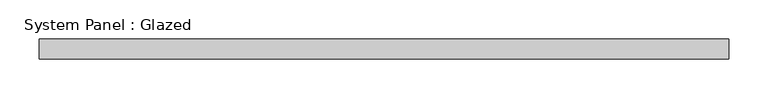
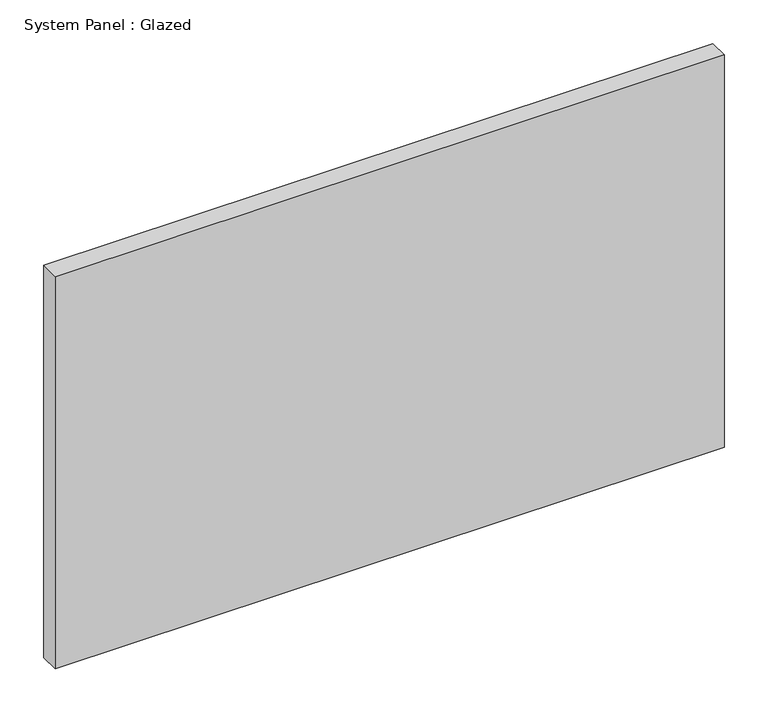
"""IFC4 building model written with IfcOpenShell, lengths in millimetres: plate geometry, System Panel : Glazed."""

from ifc_helpers import new_model, si_unit, origin, origin_with_axes, place, context, project, spatial, polyline, outline, extrude, source, transform, mapped, element, save


def system_panel_glazed_a6f8d3da(model_context):
    return source(origin(), model_context, "Body", "SweptSolid", [
        extrude(outline(polyline([(440.2666667, 19.05), (-440.2666667, 19.05), (-440.2666667, 44.45), (440.2666667, 44.45), (440.2666667, 19.05)])), origin_with_axes(), (0.0, 0.0, 1.0), 545.6538352),
    ])


if __name__ == "__main__":
    model = new_model("IFC4")
    model_context = context("Model", 3, world=origin())
    ifc_project = project(units=[si_unit("LENGTHUNIT", "METRE", prefix="MILLI")], contexts=[model_context])
    site = spatial("IfcSite", under=ifc_project)
    building = spatial("IfcBuilding", under=site)
    placement = place(None, origin())
    system_panel_glazed_shape = system_panel_glazed_a6f8d3da(model_context)
    element("IfcPlate", 1, ObjectType="System Panel : Glazed", at=placement, inside=building, context=model_context, shape_type="MappedRepresentation", body=[
        mapped(system_panel_glazed_shape, transform((0.0, 0.0, 0.0), x_axis=(1.0, 0.0, 0.0), y_axis=(0.0, 1.0, 0.0), z_axis=(0.0, 0.0, 1.0))),
    ])
    save(model, "model.ifc")

# Revit data of these elements
# Type "System Panel : Glazed"
#   Construction Type Id = "GSP4R"
#   Analytic Construction = "1/8 in Pilkington single glazing"
#   Visual Light Transmittance = 0.9
#   Solar Heat Gain Coefficient = 0.86
#   Heat Transfer Coefficient (U) = 1.18115 BTU/(h·ft²·°F)
#   Define Thermal Properties by = 1
# Element 1 (IfcPlate, "System Panel : Glazed")
#   Materials on its faces: "Glass"
# Materials
#   "Glass": class "Glass", colour RGB 0 128 192, transparency 0.75, Description = "Soda Lime Glass", Cost = 0
